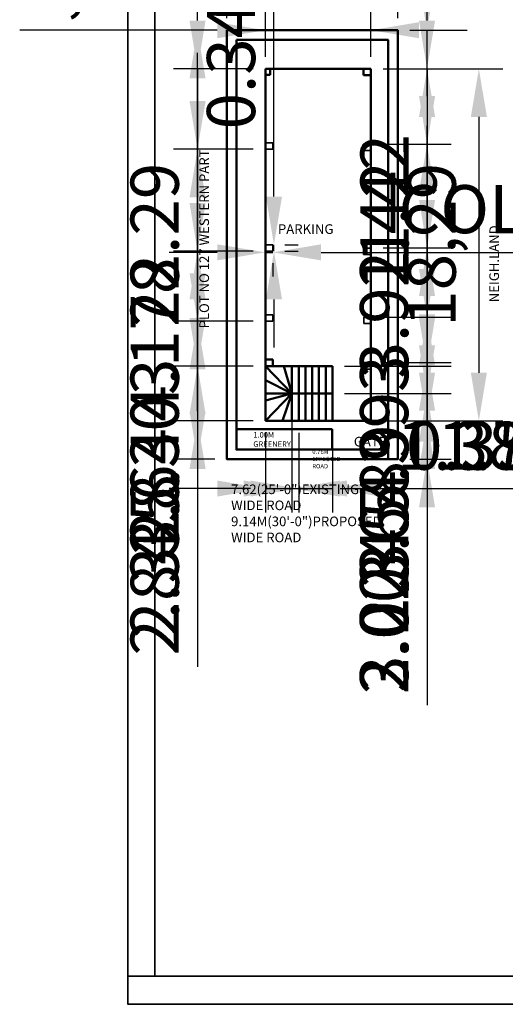
# Model space of a CAD drawing. Units: metres. Extents: x 782 to 1487, y 1262 to 7446.
# Tile 1 of 25: x 782 to 807, y 1262 to 1313. Entities that reach past the tile are written whole.
import ezdxf

# ---------------------------------------------------------------- set-up
doc = ezdxf.new("R2010")
doc.units = ezdxf.units.M
for name, color, linetype, lineweight in [('A-ANNO-DIMS', 2, 'Continuous', 18), ('A-ANNO-TEXT', 3, 'Continuous', 18), ('A-ANNO-TTLB', 7, 'Continuous', 35), ('A-AREA-IDEN', 3, 'Continuous', 18), ('A-COLS', 1, 'Continuous', 35), ('A-WALL', 7, 'Continuous', 50)]:
    doc.layers.add(name, color=color, linetype=linetype, lineweight=lineweight)
doc.styles.get("Standard").update_dxf_attribs({"font": 'arial.ttf'})
doc.dimstyles.new('ISO-25', dxfattribs={"dimtxt": 2.5, "dimasz": 2.5, "dimexe": 1.25, "dimexo": 0.625, "dimtad": 1, "dimtxsty": 'Standard', "dimcen": 2.5, "dimadec": 0, "dimazin": 0, "dimtfac": 1, "dimtmove": 0, "dimatfit": 3, "dimfxl": 1, "dimarcsym": 0})

# ---------------------------------------------------------------- blocks, each defined once
blk = doc.blocks.new('*D1')
at = {"layer": 'A-ANNO-DIMS', "color": 0, "lineweight": -2, "transparency": 16777216}
for p, q in [((800.664, 1310.946), (806.889, 1310.946)), ((805.639, 1308.446), (805.639, 1295.16)), ((800.664, 1292.66), (806.889, 1292.66))]:
    blk.add_line(p, q, dxfattribs=at)
at = {"layer": 'A-ANNO-DIMS', "color": 0, "transparency": 16777216}
for points in [[(805.222, 1308.446), (806.056, 1308.446), (805.639, 1310.946)], [(805.222, 1295.16), (806.056, 1295.16), (805.639, 1292.66)]]:
    blk.add_solid(points, dxfattribs=at)
at = {"layer": 'Defpoints', "color": 0, "transparency": 16777216}
for p in [(800.039, 1310.946), (800.039, 1292.66), (805.639, 1292.66)]:
    blk.add_point(p, dxfattribs=at)
at = {"layer": 'A-ANNO-DIMS', "color": 0, "transparency": 16777216, "insert": (803.512, 1301.803), "char_height": 2.5, "attachment_point": 5, "rotation": 90}
blk.add_mtext('18,29', dxfattribs=at)
blk = doc.blocks.new('*D2')
at = {"layer": 'A-ANNO-DIMS', "color": 0, "lineweight": -2, "transparency": 16777216}
for p, q in [((794.559, 1311.575), (794.559, 1314.2)), ((800.039, 1311.575), (800.039, 1314.2)), ((792.059, 1312.95), (781.81, 1312.95)), ((800.039, 1312.95), (794.559, 1312.95)), ((802.539, 1312.95), (805.039, 1312.95))]:
    blk.add_line(p, q, dxfattribs=at)
at = {"layer": 'A-ANNO-DIMS', "color": 0, "transparency": 16777216}
for points in [[(792.059, 1313.367), (792.059, 1312.534), (794.559, 1312.95)], [(802.539, 1313.367), (802.539, 1312.534), (800.039, 1312.95)]]:
    blk.add_solid(points, dxfattribs=at)
at = {"layer": 'Defpoints', "color": 0, "transparency": 16777216}
for p in [(794.559, 1312.95), (794.559, 1310.95), (800.039, 1310.95)]:
    blk.add_point(p, dxfattribs=at)
at = {"layer": 'A-ANNO-DIMS', "color": 0, "transparency": 16777216, "insert": (785.685, 1315.078), "char_height": 2.5, "width": 6.51678, "attachment_point": 5}
blk.add_mtext('5,48', dxfattribs=at)
blk = doc.blocks.new('COLUMN-MARK')
for p, q in [((0, 0.336), (0.387, 0.336)), ((0.387, 0.336), (0.387, 0)), ((0.387, 0), (0, 0))]:
    blk.add_line(p, q)
blk = doc.blocks.new('*D30')
at = {"layer": 'A-ANNO-DIMS', "color": 0, "lineweight": -2, "transparency": 16777216}
for p, q in [((792.059, 1301.411), (789.559, 1301.411)), ((794.559, 1301.411), (794.946, 1301.411)), ((797.446, 1301.411), (832.354, 1301.411)), ((794.559, 1300.844), (794.559, 1300.161)), ((794.946, 1300.844), (794.946, 1300.161))]:
    blk.add_line(p, q, dxfattribs=at)
at = {"layer": 'A-ANNO-DIMS', "color": 0, "transparency": 16777216}
for points in [[(792.059, 1301.827), (792.059, 1300.994), (794.559, 1301.411)], [(797.446, 1301.827), (797.446, 1300.994), (794.946, 1301.411)]]:
    blk.add_solid(points, dxfattribs=at)
at = {"layer": 'Defpoints', "color": 0, "transparency": 16777216}
for p in [(794.559, 1301.469), (794.946, 1301.469), (794.946, 1301.411)]:
    blk.add_point(p, dxfattribs=at)
at = {"layer": 'A-ANNO-DIMS', "color": 0, "transparency": 16777216, "insert": (816.15, 1303.33), "char_height": 2.5, "attachment_point": 5}
blk.add_mtext('COLUMN 0.39 TYP.', dxfattribs=at)
blk = doc.blocks.new('*D31')
at = {"layer": 'A-ANNO-DIMS', "color": 0, "lineweight": -2, "transparency": 16777216}
for p, q in [((795.004, 1304.305), (795.004, 1323.137)), ((795.004, 1301.469), (795.004, 1301.805)), ((795.571, 1301.805), (796.254, 1301.805)), ((795.571, 1301.469), (796.254, 1301.469)), ((795.004, 1298.969), (795.004, 1296.469))]:
    blk.add_line(p, q, dxfattribs=at)
at = {"layer": 'A-ANNO-DIMS', "color": 0, "transparency": 16777216}
for points in [[(794.587, 1304.305), (795.421, 1304.305), (795.004, 1301.805)], [(794.587, 1298.969), (795.421, 1298.969), (795.004, 1301.469)]]:
    blk.add_solid(points, dxfattribs=at)
at = {"layer": 'Defpoints', "color": 0, "transparency": 16777216}
for p in [(794.946, 1301.805), (794.946, 1301.469), (795.004, 1301.805)]:
    blk.add_point(p, dxfattribs=at)
at = {"layer": 'A-ANNO-DIMS', "color": 0, "transparency": 16777216, "insert": (793.102, 1314.971), "char_height": 2.5, "attachment_point": 5, "rotation": 90}
blk.add_mtext('0.34 TYP.', dxfattribs=at)
blk = doc.blocks.new('*D32')
at = {"layer": 'A-ANNO-DIMS', "color": 0, "lineweight": -2, "transparency": 16777216}
for p, q in [((791.039, 1313.45), (791.039, 1315.95)), ((793.934, 1310.95), (789.789, 1310.95)), ((791.039, 1310.95), (791.039, 1306.772)), ((793.934, 1306.772), (789.789, 1306.772)), ((791.039, 1304.272), (791.039, 1291.98))]:
    blk.add_line(p, q, dxfattribs=at)
at = {"layer": 'A-ANNO-DIMS', "color": 0, "transparency": 16777216}
for points in [[(790.622, 1313.45), (791.456, 1313.45), (791.039, 1310.95)], [(790.622, 1304.272), (791.456, 1304.272), (791.039, 1306.772)]]:
    blk.add_solid(points, dxfattribs=at)
at = {"layer": 'Defpoints', "color": 0, "transparency": 16777216}
for p in [(794.559, 1310.95), (791.039, 1306.772), (794.559, 1306.772)]:
    blk.add_point(p, dxfattribs=at)
at = {"layer": 'A-ANNO-DIMS', "color": 0, "transparency": 16777216, "insert": (789.138, 1296.876), "char_height": 2.5, "attachment_point": 5, "rotation": 90}
blk.add_mtext('4.178', dxfattribs=at)
blk = doc.blocks.new('*D33')
at = {"layer": 'A-ANNO-DIMS', "color": 0, "lineweight": -2, "transparency": 16777216}
for p, q in [((791.039, 1309.272), (791.039, 1311.772)), ((793.934, 1306.772), (789.789, 1306.772)), ((791.039, 1306.772), (791.039, 1301.469)), ((793.934, 1301.469), (789.789, 1301.469)), ((791.039, 1298.969), (791.039, 1286.783))]:
    blk.add_line(p, q, dxfattribs=at)
at = {"layer": 'A-ANNO-DIMS', "color": 0, "transparency": 16777216}
for points in [[(790.622, 1309.272), (791.456, 1309.272), (791.039, 1306.772)], [(790.622, 1298.969), (791.456, 1298.969), (791.039, 1301.469)]]:
    blk.add_solid(points, dxfattribs=at)
at = {"layer": 'Defpoints', "color": 0, "transparency": 16777216}
for p in [(794.559, 1306.772), (791.039, 1301.469), (794.559, 1301.469)]:
    blk.add_point(p, dxfattribs=at)
at = {"layer": 'A-ANNO-DIMS', "color": 0, "transparency": 16777216, "insert": (789.137, 1291.626), "char_height": 2.5, "attachment_point": 5, "rotation": 90}
blk.add_mtext('5.303', dxfattribs=at)
blk = doc.blocks.new('*D34')
at = {"layer": 'A-ANNO-DIMS', "color": 0, "lineweight": -2, "transparency": 16777216}
for p, q in [((791.039, 1303.969), (791.039, 1306.469)), ((793.934, 1301.469), (789.789, 1301.469)), ((791.039, 1301.469), (791.039, 1297.828)), ((793.934, 1297.828), (789.789, 1297.828)), ((791.039, 1295.328), (791.039, 1285.096))]:
    blk.add_line(p, q, dxfattribs=at)
at = {"layer": 'A-ANNO-DIMS', "color": 0, "transparency": 16777216}
for points in [[(790.622, 1303.969), (791.456, 1303.969), (791.039, 1301.469)], [(790.622, 1295.328), (791.456, 1295.328), (791.039, 1297.828)]]:
    blk.add_solid(points, dxfattribs=at)
at = {"layer": 'Defpoints', "color": 0, "transparency": 16777216}
for p in [(794.559, 1301.469), (791.039, 1297.828), (794.559, 1297.828)]:
    blk.add_point(p, dxfattribs=at)
at = {"layer": 'A-ANNO-DIMS', "color": 0, "transparency": 16777216, "insert": (789.137, 1288.962), "char_height": 2.5, "attachment_point": 5, "rotation": 90}
blk.add_mtext('3.64', dxfattribs=at)
blk = doc.blocks.new('*D35')
at = {"layer": 'A-ANNO-DIMS', "color": 0, "lineweight": -2, "transparency": 16777216}
for p, q in [((791.039, 1300.328), (791.039, 1302.828)), ((793.934, 1297.828), (789.789, 1297.828)), ((791.039, 1297.828), (791.039, 1295.5)), ((793.934, 1295.5), (789.789, 1295.5)), ((791.039, 1293), (791.039, 1280.766))]:
    blk.add_line(p, q, dxfattribs=at)
at = {"layer": 'A-ANNO-DIMS', "color": 0, "transparency": 16777216}
for points in [[(790.622, 1300.328), (791.456, 1300.328), (791.039, 1297.828)], [(790.622, 1293), (791.456, 1293), (791.039, 1295.5)]]:
    blk.add_solid(points, dxfattribs=at)
at = {"layer": 'Defpoints', "color": 0, "transparency": 16777216}
for p in [(794.559, 1297.828), (791.039, 1295.5), (794.559, 1295.5)]:
    blk.add_point(p, dxfattribs=at)
at = {"layer": 'A-ANNO-DIMS', "color": 0, "transparency": 16777216, "insert": (789.137, 1285.633), "char_height": 2.5, "attachment_point": 5, "rotation": 90}
blk.add_mtext('2.328', dxfattribs=at)
blk = doc.blocks.new('*D36')
at = {"layer": 'A-ANNO-DIMS', "color": 0, "lineweight": -2, "transparency": 16777216}
for p, q in [((791.039, 1298), (791.039, 1300.5)), ((793.934, 1295.5), (789.789, 1295.5)), ((791.039, 1295.5), (791.039, 1292.66)), ((793.934, 1292.66), (789.789, 1292.66)), ((791.039, 1290.16), (791.039, 1279.884))]:
    blk.add_line(p, q, dxfattribs=at)
at = {"layer": 'A-ANNO-DIMS', "color": 0, "transparency": 16777216}
for points in [[(790.622, 1298), (791.456, 1298), (791.039, 1295.5)], [(790.622, 1290.16), (791.456, 1290.16), (791.039, 1292.66)]]:
    blk.add_solid(points, dxfattribs=at)
at = {"layer": 'Defpoints', "color": 0, "transparency": 16777216}
for p in [(794.559, 1295.5), (791.039, 1292.66), (794.559, 1292.66)]:
    blk.add_point(p, dxfattribs=at)
at = {"layer": 'A-ANNO-DIMS', "color": 0, "transparency": 16777216, "insert": (789.138, 1283.772), "char_height": 2.5, "attachment_point": 5, "rotation": 90}
blk.add_mtext('2.84', dxfattribs=at)
blk = doc.blocks.new('*D37')
at = {"layer": 'A-ANNO-DIMS', "color": 0, "lineweight": -2, "transparency": 16777216}
for p, q in [((802.949, 1313.45), (802.949, 1315.95)), ((800.664, 1310.95), (804.199, 1310.95)), ((802.949, 1310.95), (802.949, 1307.03)), ((800.653, 1307.03), (804.199, 1307.03)), ((802.949, 1304.53), (802.949, 1294.314))]:
    blk.add_line(p, q, dxfattribs=at)
at = {"layer": 'A-ANNO-DIMS', "color": 0, "transparency": 16777216}
for points in [[(802.532, 1313.45), (803.366, 1313.45), (802.949, 1310.95)], [(802.532, 1304.53), (803.366, 1304.53), (802.949, 1307.03)]]:
    blk.add_solid(points, dxfattribs=at)
at = {"layer": 'Defpoints', "color": 0, "transparency": 16777216}
for p in [(800.039, 1310.95), (800.028, 1307.03), (802.949, 1307.03)]:
    blk.add_point(p, dxfattribs=at)
at = {"layer": 'A-ANNO-DIMS', "color": 0, "transparency": 16777216, "insert": (801.047, 1298.172), "char_height": 2.5, "attachment_point": 5, "rotation": 90}
blk.add_mtext('3.92', dxfattribs=at)
blk = doc.blocks.new('*D38')
at = {"layer": 'A-ANNO-DIMS', "color": 0, "lineweight": -2, "transparency": 16777216}
for p, q in [((802.949, 1309.53), (802.949, 1312.03)), ((800.653, 1307.03), (804.199, 1307.03)), ((802.949, 1307.03), (802.949, 1301.637)), ((800.666, 1301.637), (804.199, 1301.637)), ((802.949, 1299.137), (802.949, 1286.951))]:
    blk.add_line(p, q, dxfattribs=at)
at = {"layer": 'A-ANNO-DIMS', "color": 0, "transparency": 16777216}
for points in [[(802.532, 1309.53), (803.366, 1309.53), (802.949, 1307.03)], [(802.532, 1299.137), (803.366, 1299.137), (802.949, 1301.637)]]:
    blk.add_solid(points, dxfattribs=at)
at = {"layer": 'Defpoints', "color": 0, "transparency": 16777216}
for p in [(800.028, 1307.03), (800.041, 1301.637), (802.949, 1301.637)]:
    blk.add_point(p, dxfattribs=at)
at = {"layer": 'A-ANNO-DIMS', "color": 0, "transparency": 16777216, "insert": (801.047, 1291.794), "char_height": 2.5, "attachment_point": 5, "rotation": 90}
blk.add_mtext('5.393', dxfattribs=at)
blk = doc.blocks.new('*D39')
at = {"layer": 'A-ANNO-DIMS', "color": 0, "lineweight": -2, "transparency": 16777216}
for p, q in [((802.949, 1304.137), (802.949, 1306.637)), ((800.666, 1301.637), (804.199, 1301.637)), ((802.949, 1301.637), (802.949, 1298.048)), ((800.678, 1298.048), (804.199, 1298.048)), ((802.949, 1295.548), (802.949, 1283.359))]:
    blk.add_line(p, q, dxfattribs=at)
at = {"layer": 'A-ANNO-DIMS', "color": 0, "transparency": 16777216}
for points in [[(802.532, 1304.137), (803.366, 1304.137), (802.949, 1301.637)], [(802.532, 1295.548), (803.366, 1295.548), (802.949, 1298.048)]]:
    blk.add_solid(points, dxfattribs=at)
at = {"layer": 'Defpoints', "color": 0, "transparency": 16777216}
for p in [(800.041, 1301.637), (800.053, 1298.048), (802.949, 1298.048)]:
    blk.add_point(p, dxfattribs=at)
at = {"layer": 'A-ANNO-DIMS', "color": 0, "transparency": 16777216, "insert": (801.047, 1288.203), "char_height": 2.5, "attachment_point": 5, "rotation": 90}
blk.add_mtext('3.589', dxfattribs=at)
blk = doc.blocks.new('*D40')
at = {"layer": 'A-ANNO-DIMS', "color": 0, "lineweight": -2, "transparency": 16777216}
for p, q in [((802.949, 1300.548), (802.949, 1303.048)), ((800.678, 1298.048), (804.199, 1298.048)), ((802.949, 1298.048), (802.949, 1295.685)), ((800.659, 1295.685), (804.199, 1295.685)), ((802.949, 1293.185), (802.949, 1280.966))]:
    blk.add_line(p, q, dxfattribs=at)
at = {"layer": 'A-ANNO-DIMS', "color": 0, "transparency": 16777216}
for points in [[(802.532, 1300.548), (803.366, 1300.548), (802.949, 1298.048)], [(802.532, 1293.185), (803.366, 1293.185), (802.949, 1295.685)]]:
    blk.add_solid(points, dxfattribs=at)
at = {"layer": 'Defpoints', "color": 0, "transparency": 16777216}
for p in [(800.053, 1298.048), (800.034, 1295.685), (802.949, 1295.685)]:
    blk.add_point(p, dxfattribs=at)
at = {"layer": 'A-ANNO-DIMS', "color": 0, "transparency": 16777216, "insert": (801.047, 1285.825), "char_height": 2.5, "attachment_point": 5, "rotation": 90}
blk.add_mtext('2.364', dxfattribs=at)
blk = doc.blocks.new('*D41')
at = {"layer": 'A-ANNO-DIMS', "color": 0, "lineweight": -2, "transparency": 16777216}
for p, q in [((802.949, 1298.185), (802.949, 1300.685)), ((800.659, 1295.685), (804.199, 1295.685)), ((802.949, 1295.685), (802.949, 1292.66)), ((800.664, 1292.66), (804.199, 1292.66)), ((802.949, 1290.16), (802.949, 1277.986))]:
    blk.add_line(p, q, dxfattribs=at)
at = {"layer": 'A-ANNO-DIMS', "color": 0, "transparency": 16777216}
for points in [[(802.532, 1298.185), (803.366, 1298.185), (802.949, 1295.685)], [(802.532, 1290.16), (803.366, 1290.16), (802.949, 1292.66)]]:
    blk.add_solid(points, dxfattribs=at)
at = {"layer": 'Defpoints', "color": 0, "transparency": 16777216}
for p in [(800.034, 1295.685), (800.039, 1292.66), (802.949, 1292.66)]:
    blk.add_point(p, dxfattribs=at)
at = {"layer": 'A-ANNO-DIMS', "color": 0, "transparency": 16777216, "insert": (801.047, 1282.823), "char_height": 2.5, "attachment_point": 5, "rotation": 90}
blk.add_mtext('3.024', dxfattribs=at)
blk = doc.blocks.new('*D42')
at = {"layer": 'A-ANNO-DIMS', "color": 0, "lineweight": -2, "transparency": 16777216}
for p, q in [((792.559, 1313.575), (792.559, 1315.72)), ((801.429, 1313.575), (801.429, 1315.72)), ((795.059, 1314.47), (798.929, 1314.47))]:
    blk.add_line(p, q, dxfattribs=at)
at = {"layer": 'A-ANNO-DIMS', "color": 0, "transparency": 16777216}
for points in [[(795.059, 1314.887), (795.059, 1314.054), (792.559, 1314.47)], [(798.929, 1314.887), (798.929, 1314.054), (801.429, 1314.47)]]:
    blk.add_solid(points, dxfattribs=at)
at = {"layer": 'Defpoints', "color": 0, "transparency": 16777216}
for p in [(801.429, 1314.47), (792.559, 1312.95), (801.429, 1312.95)]:
    blk.add_point(p, dxfattribs=at)
at = {"layer": 'A-ANNO-DIMS', "color": 0, "transparency": 16777216, "insert": (796.994, 1316.372), "char_height": 2.5, "attachment_point": 5}
blk.add_mtext('8.87', dxfattribs=at)
blk = doc.blocks.new('*D43')
at = {"layer": 'A-ANNO-DIMS', "color": 0, "lineweight": -2, "transparency": 16777216}
for p, q in [((792.559, 1313.575), (792.559, 1315.72)), ((794.559, 1311.575), (794.559, 1315.72)), ((790.059, 1314.47), (787.559, 1314.47)), ((792.559, 1314.47), (794.559, 1314.47)), ((797.059, 1314.47), (807.337, 1314.47))]:
    blk.add_line(p, q, dxfattribs=at)
at = {"layer": 'A-ANNO-DIMS', "color": 0, "transparency": 16777216}
for points in [[(790.059, 1314.887), (790.059, 1314.054), (792.559, 1314.47)], [(797.059, 1314.887), (797.059, 1314.054), (794.559, 1314.47)]]:
    blk.add_solid(points, dxfattribs=at)
at = {"layer": 'Defpoints', "color": 0, "transparency": 16777216}
for p in [(794.559, 1314.47), (792.559, 1312.95), (794.559, 1310.95)]:
    blk.add_point(p, dxfattribs=at)
at = {"layer": 'A-ANNO-DIMS', "color": 0, "transparency": 16777216, "insert": (803.448, 1316.372), "char_height": 2.5, "attachment_point": 5}
blk.add_mtext('2.00', dxfattribs=at)
blk = doc.blocks.new('*D44')
at = {"layer": 'A-ANNO-DIMS', "color": 0, "lineweight": -2, "transparency": 16777216}
for p, q in [((800.039, 1311.575), (800.039, 1315.72)), ((801.429, 1313.575), (801.429, 1315.72)), ((797.539, 1314.47), (795.039, 1314.47)), ((800.039, 1314.47), (801.429, 1314.47)), ((803.929, 1314.47), (813.943, 1314.47))]:
    blk.add_line(p, q, dxfattribs=at)
at = {"layer": 'A-ANNO-DIMS', "color": 0, "transparency": 16777216}
for points in [[(797.539, 1314.887), (797.539, 1314.054), (800.039, 1314.47)], [(803.929, 1314.887), (803.929, 1314.054), (801.429, 1314.47)]]:
    blk.add_solid(points, dxfattribs=at)
at = {"layer": 'Defpoints', "color": 0, "transparency": 16777216}
for p in [(801.429, 1314.47), (801.429, 1312.95), (800.039, 1310.95)]:
    blk.add_point(p, dxfattribs=at)
at = {"layer": 'A-ANNO-DIMS', "color": 0, "transparency": 16777216, "insert": (810.186, 1316.373), "char_height": 2.5, "attachment_point": 5}
blk.add_mtext('1.39', dxfattribs=at)
blk = doc.blocks.new('*D45')
at = {"layer": 'A-ANNO-DIMS', "color": 0, "lineweight": -2, "transparency": 16777216}
for p, q in [((791.934, 1312.95), (789.789, 1312.95)), ((791.039, 1293.16), (791.039, 1310.45)), ((791.934, 1290.66), (789.789, 1290.66))]:
    blk.add_line(p, q, dxfattribs=at)
at = {"layer": 'A-ANNO-DIMS', "color": 0, "transparency": 16777216}
for points in [[(790.622, 1310.45), (791.456, 1310.45), (791.039, 1312.95)], [(790.622, 1293.16), (791.456, 1293.16), (791.039, 1290.66)]]:
    blk.add_solid(points, dxfattribs=at)
at = {"layer": 'Defpoints', "color": 0, "transparency": 16777216}
for p in [(791.039, 1312.95), (792.559, 1312.95), (792.559, 1290.66)]:
    blk.add_point(p, dxfattribs=at)
at = {"layer": 'A-ANNO-DIMS', "color": 0, "transparency": 16777216, "insert": (789.138, 1301.805), "char_height": 2.5, "attachment_point": 5, "rotation": 90}
blk.add_mtext('22.29', dxfattribs=at)
blk = doc.blocks.new('*D46')
at = {"layer": 'A-ANNO-DIMS', "color": 0, "lineweight": -2, "transparency": 16777216}
for p, q in [((802.949, 1295.16), (802.949, 1297.66)), ((800.664, 1292.66), (804.199, 1292.66)), ((802.949, 1292.66), (802.949, 1290.66)), ((802.054, 1290.66), (804.199, 1290.66)), ((802.949, 1288.16), (802.949, 1277.882))]:
    blk.add_line(p, q, dxfattribs=at)
at = {"layer": 'A-ANNO-DIMS', "color": 0, "transparency": 16777216}
for points in [[(802.532, 1295.16), (803.366, 1295.16), (802.949, 1292.66)], [(802.532, 1288.16), (803.366, 1288.16), (802.949, 1290.66)]]:
    blk.add_solid(points, dxfattribs=at)
at = {"layer": 'Defpoints', "color": 0, "transparency": 16777216}
for p in [(800.039, 1292.66), (801.429, 1290.66), (802.949, 1290.66)]:
    blk.add_point(p, dxfattribs=at)
at = {"layer": 'A-ANNO-DIMS', "color": 0, "transparency": 16777216, "insert": (801.048, 1281.771), "char_height": 2.5, "attachment_point": 5, "rotation": 90}
blk.add_mtext('2.00', dxfattribs=at)
blk = doc.blocks.new('*D47')
at = {"layer": 'A-ANNO-DIMS', "color": 0, "lineweight": -2, "transparency": 16777216}
for p, q in [((802.949, 1315.45), (802.949, 1325.728)), ((802.054, 1312.95), (804.199, 1312.95)), ((802.949, 1310.95), (802.949, 1312.95)), ((800.664, 1310.95), (804.199, 1310.95)), ((802.949, 1308.45), (802.949, 1305.95))]:
    blk.add_line(p, q, dxfattribs=at)
at = {"layer": 'A-ANNO-DIMS', "color": 0, "transparency": 16777216}
for points in [[(802.532, 1315.45), (803.366, 1315.45), (802.949, 1312.95)], [(802.532, 1308.45), (803.366, 1308.45), (802.949, 1310.95)]]:
    blk.add_solid(points, dxfattribs=at)
at = {"layer": 'Defpoints', "color": 0, "transparency": 16777216}
for p in [(801.429, 1312.95), (802.949, 1312.95), (800.039, 1310.95)]:
    blk.add_point(p, dxfattribs=at)
at = {"layer": 'A-ANNO-DIMS', "color": 0, "transparency": 16777216, "insert": (801.048, 1321.839), "char_height": 2.5, "attachment_point": 5, "rotation": 90}
blk.add_mtext('2.00', dxfattribs=at)
blk = doc.blocks.new('*D48')
at = {"layer": 'A-ANNO-DIMS', "color": 0, "lineweight": -2, "transparency": 16777216}
for p, q in [((795.937, 1293.455), (795.937, 1287.89)), ((794.559, 1292.035), (794.559, 1287.89)), ((792.059, 1289.14), (789.559, 1289.14)), ((794.559, 1289.14), (795.937, 1289.14)), ((798.437, 1289.14), (808.45, 1289.14))]:
    blk.add_line(p, q, dxfattribs=at)
at = {"layer": 'A-ANNO-DIMS', "color": 0, "transparency": 16777216}
for points in [[(792.059, 1289.557), (792.059, 1288.724), (794.559, 1289.14)], [(798.437, 1289.557), (798.437, 1288.724), (795.937, 1289.14)]]:
    blk.add_solid(points, dxfattribs=at)
at = {"layer": 'Defpoints', "color": 0, "transparency": 16777216}
for p in [(795.937, 1294.08), (794.559, 1292.66), (795.937, 1289.14)]:
    blk.add_point(p, dxfattribs=at)
at = {"layer": 'A-ANNO-DIMS', "color": 0, "transparency": 16777216, "insert": (804.694, 1291.043), "char_height": 2.5, "attachment_point": 5}
blk.add_mtext('1.38', dxfattribs=at)
blk = doc.blocks.new('*D49')
at = {"layer": 'A-ANNO-DIMS', "color": 0, "lineweight": -2, "transparency": 16777216}
for p, q in [((795.937, 1292.035), (795.937, 1287.89)), ((796.288, 1292.035), (796.288, 1287.89)), ((793.437, 1289.14), (790.937, 1289.14)), ((795.937, 1289.14), (796.288, 1289.14)), ((798.788, 1289.14), (809.051, 1289.14))]:
    blk.add_line(p, q, dxfattribs=at)
at = {"layer": 'A-ANNO-DIMS', "color": 0, "transparency": 16777216}
for points in [[(793.437, 1289.557), (793.437, 1288.724), (795.937, 1289.14)], [(798.788, 1289.557), (798.788, 1288.724), (796.288, 1289.14)]]:
    blk.add_solid(points, dxfattribs=at)
at = {"layer": 'Defpoints', "color": 0, "transparency": 16777216}
for p in [(795.937, 1292.66), (796.288, 1292.66), (796.288, 1289.14)]:
    blk.add_point(p, dxfattribs=at)
at = {"layer": 'A-ANNO-DIMS', "color": 0, "transparency": 16777216, "insert": (805.169, 1291.043), "char_height": 2.5, "attachment_point": 5}
blk.add_mtext('0.35', dxfattribs=at)
blk = doc.blocks.new('*D50')
at = {"layer": 'A-ANNO-DIMS', "color": 0, "lineweight": -2, "transparency": 16777216}
for p, q in [((796.288, 1292.035), (796.288, 1287.89)), ((798.044, 1292.035), (798.044, 1287.89)), ((793.788, 1289.14), (791.288, 1289.14)), ((796.288, 1289.14), (798.044, 1289.14)), ((800.544, 1289.14), (810.551, 1289.14))]:
    blk.add_line(p, q, dxfattribs=at)
at = {"layer": 'A-ANNO-DIMS', "color": 0, "transparency": 16777216}
for points in [[(793.788, 1289.557), (793.788, 1288.724), (796.288, 1289.14)], [(800.544, 1289.557), (800.544, 1288.724), (798.044, 1289.14)]]:
    blk.add_solid(points, dxfattribs=at)
at = {"layer": 'Defpoints', "color": 0, "transparency": 16777216}
for p in [(796.288, 1292.66), (798.044, 1292.66), (798.044, 1289.14)]:
    blk.add_point(p, dxfattribs=at)
at = {"layer": 'A-ANNO-DIMS', "color": 0, "transparency": 16777216, "insert": (806.798, 1291.042), "char_height": 2.5, "attachment_point": 5}
blk.add_mtext('1.76', dxfattribs=at)
blk = doc.blocks.new('*D51')
at = {"layer": 'A-ANNO-DIMS', "color": 0, "lineweight": -2, "transparency": 16777216}
for p, q in [((802.949, 1296.58), (802.949, 1306.563)), ((798.669, 1294.08), (804.199, 1294.08)), ((802.949, 1292.66), (802.949, 1294.08)), ((798.669, 1292.66), (804.199, 1292.66)), ((802.949, 1290.16), (802.949, 1287.66))]:
    blk.add_line(p, q, dxfattribs=at)
at = {"layer": 'A-ANNO-DIMS', "color": 0, "transparency": 16777216}
for points in [[(802.532, 1296.58), (803.366, 1296.58), (802.949, 1294.08)], [(802.532, 1290.16), (803.366, 1290.16), (802.949, 1292.66)]]:
    blk.add_solid(points, dxfattribs=at)
at = {"layer": 'Defpoints', "color": 0, "transparency": 16777216}
for p in [(798.044, 1294.08), (802.949, 1294.08), (798.044, 1292.66)]:
    blk.add_point(p, dxfattribs=at)
at = {"layer": 'A-ANNO-DIMS', "color": 0, "transparency": 16777216, "insert": (801.069, 1302.822), "char_height": 2.5, "attachment_point": 5, "rotation": 90}
blk.add_mtext('1.42', dxfattribs=at)
blk = doc.blocks.new('*D52')
at = {"layer": 'A-ANNO-DIMS', "color": 0, "lineweight": -2, "transparency": 16777216}
for p, q in [((802.949, 1298), (802.949, 1307.983)), ((798.669, 1295.5), (804.199, 1295.5)), ((802.949, 1294.08), (802.949, 1295.5)), ((798.669, 1294.08), (804.199, 1294.08)), ((802.949, 1291.58), (802.949, 1289.08))]:
    blk.add_line(p, q, dxfattribs=at)
at = {"layer": 'A-ANNO-DIMS', "color": 0, "transparency": 16777216}
for points in [[(802.532, 1298), (803.366, 1298), (802.949, 1295.5)], [(802.532, 1291.58), (803.366, 1291.58), (802.949, 1294.08)]]:
    blk.add_solid(points, dxfattribs=at)
at = {"layer": 'Defpoints', "color": 0, "transparency": 16777216}
for p in [(798.044, 1295.5), (802.949, 1295.5), (798.044, 1294.08)]:
    blk.add_point(p, dxfattribs=at)
at = {"layer": 'A-ANNO-DIMS', "color": 0, "transparency": 16777216, "insert": (801.069, 1304.242), "char_height": 2.5, "attachment_point": 5, "rotation": 90}
blk.add_mtext('1.42', dxfattribs=at)

msp = doc.modelspace()

# ---------------------------------------------------------------- linework, layer by layer
at = {"layer": 'A-ANNO-TTLB'}
for points in [[(787.4248, 1342.9861), (880.8003, 1342.9861), (880.8003, 1263.8004), (787.4248, 1263.8004)], [(883.6865, 1262.3458), (787.4248, 1262.3458), (787.4248, 1342.9861), (883.6865, 1342.9861)], [(788.8147, 1341.5907), (880.8003, 1341.5907), (880.8003, 1263.8004), (788.8147, 1263.8004)]]:
    msp.add_lwpolyline(points, close=True, dxfattribs=at)
at = {"layer": 'A-WALL'}
for p, q in [((793.059, 1312.4503), (793.059, 1292.6603)), ((800.929, 1312.4503), (793.059, 1312.4503)), ((800.929, 1292.6603), (800.929, 1312.4503)), ((800.039, 1310.9503), (794.559, 1310.9503)), ((794.559, 1310.9503), (794.559, 1292.6603)), ((794.559, 1310.9503), (800.039, 1310.9503)), ((794.559, 1310.9503), (794.8118, 1310.9503)), ((794.8118, 1310.9503), (794.559, 1310.9503)), ((794.8118, 1310.6369), (794.559, 1310.6369)), ((794.8118, 1310.9503), (794.8118, 1310.6369)), ((799.6518, 1310.6098), (799.6518, 1310.9464)), ((799.6518, 1310.9464), (800.0387, 1310.9464)), ((800.0387, 1310.6098), (799.6518, 1310.6098)), ((800.039, 1292.6603), (800.039, 1310.9503)), ((800.039, 1292.6603), (800.039, 1310.9503)), ((794.559, 1295.8367), (794.9459, 1295.8367)), ((794.9459, 1295.8367), (794.9459, 1295.5001)), ((794.9459, 1295.5001), (794.559, 1295.5001)), ((794.559, 1295.5001), (797.3143, 1295.5001)), ((795.9367, 1294.0802), (794.559, 1295.5001)), ((795.9367, 1295.5001), (795.5111, 1295.5001)), ((795.5111, 1295.5001), (795.9367, 1294.0802)), ((795.9367, 1295.5001), (795.9367, 1292.6603)), ((795.9367, 1294.0802), (795.9367, 1295.5001)), ((795.9367, 1292.6603), (795.9367, 1295.5001)), ((795.9367, 1294.0802), (795.9367, 1295.5001)), ((796.2879, 1294.0802), (796.2879, 1295.5001)), ((796.6392, 1294.0802), (796.6392, 1295.5001)), ((796.9904, 1294.0802), (796.9904, 1295.5001)), ((797.3143, 1295.5001), (798.0441, 1295.5001)), ((797.3416, 1294.0802), (797.3416, 1295.5001)), ((797.6929, 1294.0802), (797.6929, 1295.5001)), ((798.0441, 1295.5001), (798.0441, 1292.6603)), ((798.0441, 1294.0802), (798.0441, 1295.5001)), ((794.559, 1292.6603), (794.559, 1294.7632)), ((794.559, 1294.7632), (795.9367, 1294.0802)), ((795.9367, 1294.0802), (794.559, 1294.0802)), ((795.9367, 1294.0802), (794.559, 1294.0802)), ((795.9367, 1294.0802), (794.559, 1292.6603)), ((795.9367, 1294.0802), (794.559, 1292.6603)), ((795.9367, 1294.0802), (794.559, 1293.7117)), ((795.4461, 1292.6603), (795.9367, 1294.0802)), ((795.9367, 1294.0802), (798.0441, 1294.0802)), ((795.9367, 1294.0802), (798.0441, 1294.0802)), ((795.9367, 1294.0802), (795.9367, 1292.6603)), ((795.9367, 1294.0802), (795.9367, 1292.6603)), ((796.2879, 1294.0802), (796.2879, 1292.6603)), ((796.6392, 1294.0802), (796.6392, 1292.6603)), ((796.9904, 1294.0802), (796.9904, 1292.6603)), ((797.3416, 1294.0802), (797.3416, 1292.6603)), ((797.6929, 1294.0802), (797.6929, 1292.6603)), ((793.059, 1292.6603), (793.059, 1291.1603)), ((793.059, 1292.6603), (793.059, 1292.2252)), ((794.559, 1292.6603), (800.039, 1292.6603)), ((794.559, 1292.6603), (799.149, 1292.6603)), ((794.559, 1292.6603), (800.039, 1292.6603)), ((794.559, 1292.6603), (797.3143, 1292.6603)), ((795.9367, 1292.6603), (795.4461, 1292.6603)), ((797.3143, 1292.6603), (798.0441, 1292.6603)), ((800.929, 1291.1603), (800.929, 1292.6603)), ((793.059, 1292.2252), (798.0245, 1292.2252)), ((798.0245, 1292.2252), (798.0245, 1291.1603)), ((793.059, 1291.1603), (800.929, 1291.1603)), ((800.929, 1291.233), (800.517, 1291.233)), ((800.517, 1291.233), (800.517, 1291.1603)), ((800.929, 1291.1603), (800.929, 1291.233)), ((800.929, 1291.1603), (800.929, 1290.6603))]:
    msp.add_line(p, q, dxfattribs=at)
for points in [[(792.559, 1312.9503), (801.429, 1312.9503), (801.429, 1290.6603), (792.559, 1290.6603)], [(793.059, 1312.4503), (800.929, 1312.4503), (800.929, 1291.1603), (793.059, 1291.1603)]]:
    msp.add_lwpolyline(points, close=True, dxfattribs=at)

# ---------------------------------------------------------------- block references
at = {"layer": 'A-COLS'}
for p in [(794.559, 1306.7722), (794.559, 1301.469), (794.559, 1297.8286)]:
    msp.add_blockref('COLUMN-MARK', p, dxfattribs=at)
at = {"layer": 'A-COLS', "rotation": 180}
for p in [(800.0279, 1307.0302), (800.0411, 1301.6368), (800.0526, 1298.048), (800.0341, 1295.6843)]:
    msp.add_blockref('COLUMN-MARK', p, dxfattribs=at)

# ---------------------------------------------------------------- texts
at = {"layer": 'A-ANNO-TEXT', "char_height": 0.5, "attachment_point": 1, "rotation": 90}
for s, width, insert in [('PLOT NO 127 WESTERN PART', 13.280177, (791.1346, 1297.459)), ('NEIGH.LAND', 7.994851, (806.1821, 1298.8163))]:
    msp.add_mtext_dynamic_manual_height_columns(s, width=width, gutter_width=12.5, heights=[0], dxfattribs=dict(at, insert=insert))
at = {"layer": 'A-ANNO-TEXT', "attachment_point": 1}
for s, width, gutter_width, insert, char_height in [('1.00M GREENERY ', 1.868468, 7.1702, (793.9332, 1292.0727), 0.28681), ('\\PGATE', 1.863436, 12.5, (799.149, 1292.6603), 0.5), ('0.76M EFFECTED ROAD', 0.958525, 5.5983, (796.994, 1291.1603), 0.223933), ('\\P7.62(25\'-0")EXISTING WIDE ROAD\\P9.14M(30\'-0")PROPOSED WIDE ROAD', 4.745872, 12.5, (792.7805, 1290.1846), 0.5)]:
    msp.add_mtext_dynamic_manual_height_columns(s, width=width, gutter_width=gutter_width, heights=[0], dxfattribs=dict(at, insert=insert, char_height=char_height))
at = {"layer": 'A-AREA-IDEN', "insert": (795.2102, 1303.7032), "char_height": 0.5, "attachment_point": 1}
msp.add_mtext_dynamic_manual_height_columns('\\PPARKING', width=4.107799, gutter_width=12.5, heights=[0], dxfattribs=at)

# ---------------------------------------------------------------- dimensions: what is measured, and where the dimension line sits
at = {"layer": 'A-ANNO-DIMS'}
for base, p1, p2, override, picture, middle in [((802.949, 1312.9503), (800.039, 1310.9503), (801.429, 1312.9503), {"dimdec": 2, "dimlfac": 1, "dimrnd": 0, "dimzin": 0, "dimdsep": 46, "dimlunit": 2}, '*D47', (801.0476, 1321.8393)), ((791.039, 1306.772), (794.559, 1310.9503), (794.559, 1306.772), {"dimdec": 3, "dimlfac": 1, "dimrnd": 0, "dimzin": 0, "dimdsep": 46, "dimlunit": 2}, '*D32', (789.1376, 1296.876)), ((802.949, 1307.0305), (800.039, 1310.9503), (800.0278, 1307.0305), {"dimdec": 2, "dimlfac": 1, "dimrnd": 0, "dimzin": 0, "dimdsep": 46, "dimlunit": 2}, '*D37', (801.0468, 1298.1722)), ((791.039, 1312.9503), (792.559, 1290.6603), (792.559, 1312.9503), {"dimdec": 2, "dimlfac": 1, "dimrnd": 0, "dimzin": 0, "dimdsep": 46, "dimlunit": 2}, '*D45', (789.1376, 1301.8053)), ((791.039, 1301.4687), (794.559, 1306.772), (794.559, 1301.4687), {"dimdec": 3, "dimlfac": 1, "dimrnd": 0, "dimzin": 0, "dimdsep": 46, "dimlunit": 2}, '*D33', (789.1368, 1291.6256)), ((802.94905, 1301.63703), (800.02781, 1307.03049), (800.04103, 1301.63703), {"dimdec": 3, "dimlfac": 1, "dimrnd": 0, "dimzin": 0, "dimdsep": 46, "dimlunit": 2}, '*D38', (801.04676, 1291.79392)), ((805.6391, 1292.6603), (800.0387, 1310.9464), (800.0387, 1292.6603), {"dimclrd": 0, "dimclre": 0, "dimclrt": 0}, '*D1', (803.5117, 1301.8034)), ((802.949, 1295.5001), (798.0441, 1294.0802), (798.0441, 1295.5001), {"dimdec": 2, "dimlfac": 1, "dimrnd": 0, "dimzin": 0, "dimdsep": 46, "dimlunit": 2}, '*D52', (801.0689, 1304.2416)), ((791.039, 1297.8284), (794.559, 1301.4687), (794.559, 1297.8284), {"dimdec": 2, "dimlfac": 1, "dimrnd": 0, "dimzin": 0, "dimdsep": 46, "dimlunit": 2}, '*D34', (789.1368, 1288.9624)), ((802.949, 1294.0802), (798.0441, 1292.6603), (798.0441, 1294.0802), {"dimdec": 2, "dimlfac": 1, "dimrnd": 0, "dimzin": 0, "dimdsep": 46, "dimlunit": 2}, '*D51', (801.0689, 1302.8217)), ((802.949, 1298.0483), (800.041, 1301.637), (800.0526, 1298.0483), {"dimdec": 3, "dimlfac": 1, "dimrnd": 0, "dimzin": 0, "dimdsep": 46, "dimlunit": 2}, '*D39', (801.0468, 1288.2035)), ((802.949, 1295.6845), (800.0526, 1298.0483), (800.034, 1295.6845), {"dimdec": 3, "dimlfac": 1, "dimrnd": 0, "dimzin": 0, "dimdsep": 46, "dimlunit": 2}, '*D40', (801.0468, 1285.8252)), ((791.039, 1295.5001), (794.559, 1297.8284), (794.559, 1295.5001), {"dimdec": 3, "dimlfac": 1, "dimrnd": 0, "dimzin": 0, "dimdsep": 46, "dimlunit": 2}, '*D35', (789.1368, 1285.6332)), ((791.039, 1292.6603), (794.559, 1295.5001), (794.559, 1292.6603), {"dimdec": 2, "dimlfac": 1, "dimrnd": 0, "dimzin": 0, "dimdsep": 46, "dimlunit": 2}, '*D36', (789.1376, 1283.7722)), ((802.949, 1292.6603), (800.034, 1295.6845), (800.039, 1292.6603), {"dimdec": 3, "dimlfac": 1, "dimrnd": 0, "dimzin": 0, "dimdsep": 46, "dimlunit": 2}, '*D41', (801.0468, 1282.8232)), ((802.949, 1290.6603), (800.039, 1292.6603), (801.429, 1290.6603), {"dimdec": 2, "dimlfac": 1, "dimrnd": 0, "dimzin": 0, "dimdsep": 46, "dimlunit": 2}, '*D46', (801.0476, 1281.7713))]:
    dim = msp.add_linear_dim(base=base, p1=p1, p2=p2, angle=90, dimstyle='ISO-25', override=override, dxfattribs=at)
    dim.commit()
    dim.dimension.update_dxf_attribs({"geometry": picture, "text_midpoint": middle})
dim = msp.add_linear_dim(base=(795.004, 1301.8053), p1=(794.9459, 1301.4687), p2=(794.9459, 1301.8053), angle=90, text='<> TYP.', dimstyle='ISO-25', override={"dimdec": 2, "dimlfac": 1, "dimrnd": 0, "dimzin": 0, "dimdsep": 46, "dimlunit": 2}, dxfattribs=at)
dim.commit()
dim.dimension.update_dxf_attribs({"geometry": '*D31', "text_midpoint": (793.1017, 1314.9712)})
for base, p1, p2, override, picture, middle in [((794.559, 1314.4703), (792.559, 1312.9503), (794.559, 1310.9503), {"dimdec": 2, "dimlfac": 1, "dimrnd": 0, "dimzin": 0, "dimdsep": 46, "dimlunit": 2}, '*D43', (803.448, 1316.3718)), ((801.429, 1314.4703), (792.559, 1312.9503), (801.429, 1312.9503), {"dimdec": 2, "dimlfac": 1, "dimrnd": 0, "dimzin": 0, "dimdsep": 46, "dimlunit": 2}, '*D42', (796.994, 1316.3718)), ((801.429, 1314.4703), (800.039, 1310.9503), (801.429, 1312.9503), {"dimdec": 2, "dimlfac": 1, "dimrnd": 0, "dimzin": 0, "dimdsep": 46, "dimlunit": 2}, '*D44', (810.1859, 1316.3726)), ((794.559, 1312.9503), (800.039, 1310.9503), (794.559, 1310.9503), {"dimclrd": 0, "dimclre": 0, "dimclrt": 0}, '*D2', (785.6846, 1315.0777)), ((795.9367, 1289.1403), (794.559, 1292.6603), (795.9367, 1294.0802), {"dimdec": 2, "dimlfac": 1, "dimrnd": 0, "dimzin": 0, "dimdsep": 46, "dimlunit": 2}, '*D48', (804.6935, 1291.0426)), ((796.2879, 1289.1403), (795.9367, 1292.6603), (796.2879, 1292.6603), {"dimdec": 2, "dimlfac": 1, "dimrnd": 0, "dimzin": 0, "dimdsep": 46, "dimlunit": 2}, '*D49', (805.1692, 1291.0426)), ((798.0441, 1289.1403), (796.2879, 1292.6603), (798.0441, 1292.6603), {"dimdec": 2, "dimlfac": 1, "dimrnd": 0, "dimzin": 0, "dimdsep": 46, "dimlunit": 2}, '*D50', (806.7975, 1291.0418))]:
    dim = msp.add_linear_dim(base=base, p1=p1, p2=p2, dimstyle='ISO-25', override=override, dxfattribs=at)
    dim.commit()
    dim.dimension.update_dxf_attribs({"geometry": picture, "text_midpoint": middle})
dim = msp.add_linear_dim(base=(794.9459, 1301.4107), p1=(794.559, 1301.4687), p2=(794.9459, 1301.4687), text='COLUMN <> TYP.', dimstyle='ISO-25', override={"dimdec": 2, "dimlfac": 1, "dimrnd": 0, "dimzin": 0, "dimdsep": 46, "dimlunit": 2}, dxfattribs=at)
dim.commit()
dim.dimension.update_dxf_attribs({"geometry": '*D30', "text_midpoint": (816.1499, 1303.33)})

doc.saveas('drawing.dxf')
